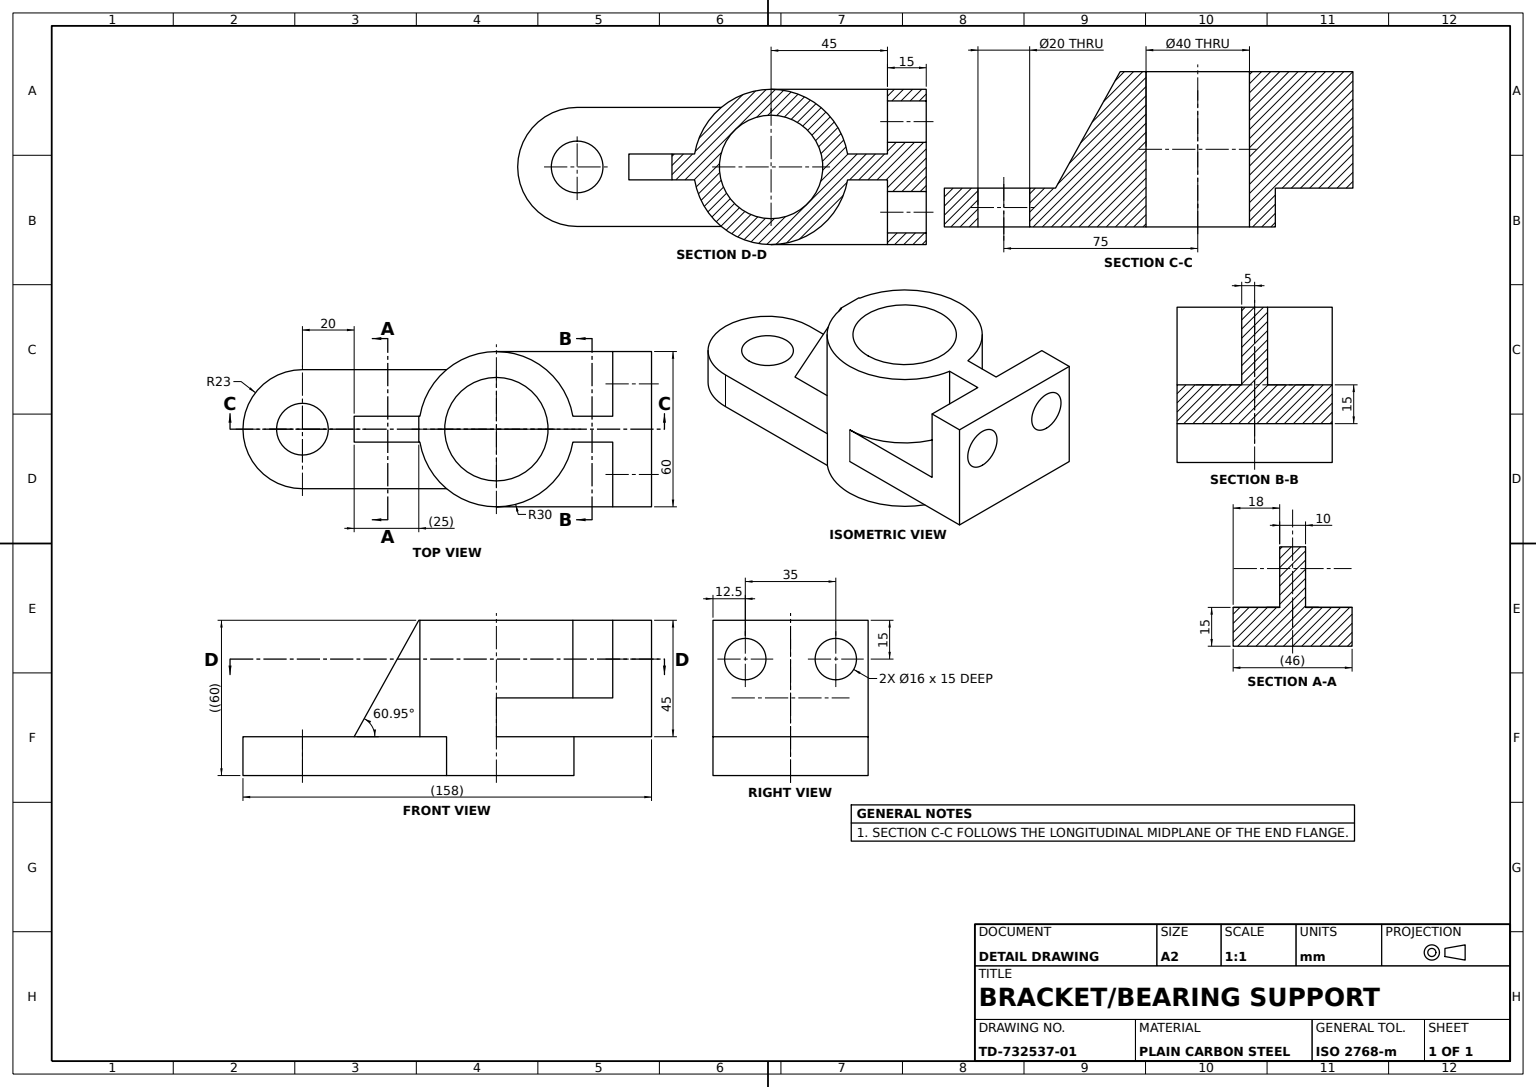
SolidWorks part; units mm, degrees
material "Plain Carbon Steel"
ref_plane "Front Plane" through (0, 0, 0) normal (0, 0, 1) x (1, 0, 0)
ref_plane "Top Plane" through (0, 0, 0) normal (0, 1, 0) x (1, 0, 0)
ref_plane "Right Plane" through (0, 0, 0) normal (1, 0, 0) x (0, 0, -1)
sketch "Bracket Body Sketch" plane through (0, 0, 0) normal (0, 0, 1) x (1, 0, 0)
  line L3 (-60, 15) -> (-60, 60)
  line L7 (-60, 60) -> (-45, 60)
  line L8 (-45, 60) -> (-45, 30)
  line L9 (-45, 30) -> (0, 30)
  line L10 (0, 30) -> (0, 15)
  line L12 (0, 0) -> (75, 0)
  line L13 (75, 0) -> (75, 15)
  line L14 (75, 15) -> (0, 15)
  line L16 (-60, 15) -> (0, 15)
  line L17 (0, 15) -> (0, 0)
  dimension "D1" = 45
  dimension "D2" = 15
  dimension "D3" = 75
  dimension "D4" = 60
  dimension "D5" = 30
  dimension "D7" = 15
extrude "Bracket Body" add sketch "Bracket Body Sketch" along normal mid plane 60 contours L3 L16 L10 L9 L8 L7 | L14 L17 L12 L13
sketch "Column Bore Sketch" plane through (0, 0, 0) normal (0, 1, 0) x (1, 0, 0)
  circle A1 centre (0, 0) radius 20
  dimension "D2" = 40
extrude "Column Bore Ø40" cut sketch "Column Bore Sketch" along normal blind 60
sketch "Column Boss Sketch" plane through (0, 0, 0) normal (0, 1, 0) x (1, 0, 0)
  circle A0 centre (0, 0) radius 20
  circle A1 centre (0, 0) radius 30
  dimension "D1" = 40
  dimension "D2" = 60
extrude "Column Boss Ø60" add sketch "Column Boss Sketch" along normal blind 60
sketch "Base Collar Sketch" plane through (0, 0, 0) normal (0, 1, 0) x (1, 0, 0)
  line L0 (75, -30) -> (75, 30) construction
  circle A0 centre (75, 0) radius 23
  dimension "D1" = 46
extrude "Base Collar Ø46" add sketch "Base Collar Sketch" along normal blind 15
sketch "Body Trim Cut Sketch" plane through (0, 15, 0) normal (0, 1, 0) x (1, 0, 0)
  line L0 (75, 23) -> (19.2614, 23)
  line L1 (75, 23) -> (75, 30)
  line L2 (75, 30) -> (0, 30)
  line L3 (75, 30) -> (0, 30) construction
  line L4 (0, 0) -> (58.0662, 0) construction
  line L5 (75, -23) -> (75, -30)
  line L6 (75, -30) -> (0, -30)
  line L7 (75, -23) -> (19.2614, -23)
  circle A0 centre (75, 0) radius 10
  circle A1 centre (0, 0) radius 30 construction
  arc A2 (0, -30) -> (19.2614, -23) centre (0, 0) ccw
  arc A3 (19.2614, 23) -> (0, 30) centre (0, 0) ccw
  dimension "D1" = 20
extrude "Body Trim Cut" cut sketch "Body Trim Cut Sketch" against normal through all
sketch "Side Block Cut Sketch" plane through (-45, 0, 0) normal (1, 0, 0) x (0, 0, -1)
  line L0 (0, 60) -> (0, 30) construction
  line L1 (-30, 60) -> (30, 60) construction
  line L2 (-30, 30) -> (30, 30) construction
  line L3 (0, 45) -> (-17.5, 45) construction
  line L4 (-17.5, 45) -> (-17.5, 60) construction
  circle A0 centre (-17.5, 45) radius 8
  circle A1 centre (17.5, 45) radius 8
  dimension "D1" = 16
  dimension "D2" = 17.5
extrude "Side Block Cut" cut sketch "Side Block Cut Sketch" against normal through all
sketch "Pad Boss Sketch" plane through (-45, 0, 0) normal (1, 0, 0) x (0, 0, -1)
  line L0 (0, 60) -> (5, 60)
  line L1 (-30, 60) -> (30, 60) construction
  line L2 (5, 60) -> (5, 30)
  line L3 (-30, 30) -> (30, 30) construction
  line L4 (5, 30) -> (-5, 30)
  line L5 (-5, 30) -> (-5, 60)
  line L6 (-5, 60) -> (0, 60)
  dimension "D1" = 5
  dimension "D2" = 5
extrude "Pad Boss 18mm" add sketch "Pad Boss Sketch" along normal blind 18
sketch "Support Rib Sketch" plane through (0, 0, 0) normal (0, 0, 1) x (1, 0, 0)
  line L1 (30, 15) -> (30, 60) construction
  line L2 (75, 15) -> (19.2614, 15) construction
  line L3 (30, 15) -> (55, 15)
  line L4 (55, 15) -> (30, 60)
  line L5 (30, 60) -> (20, 60)
  line L6 (30, 60) -> (-29.5804, 60) construction
  line L8 (20, 60) -> (20, 15)
  line L9 (20, 15) -> (30, 15)
  dimension "D1" = 25
  dimension "D2" = 10
extrude "Support Rib" add sketch "Support Rib Sketch" along normal mid plane 10
